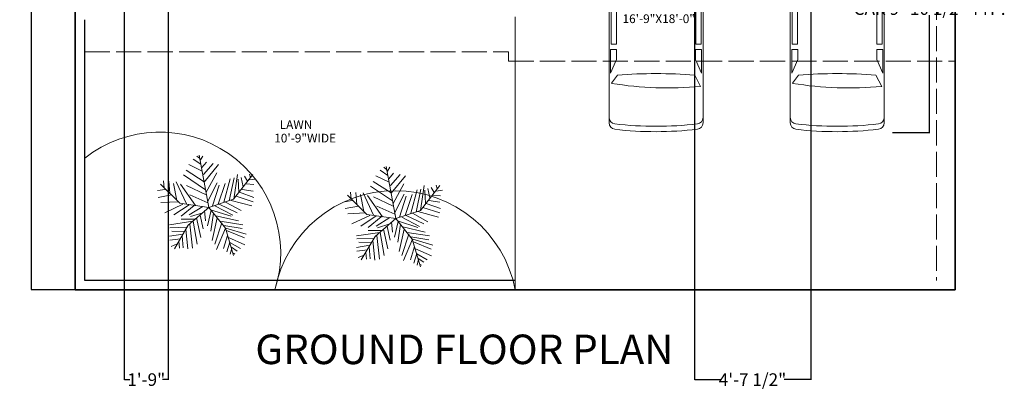
# Model space of a CAD drawing. Units: inches. Extents: x 79 to 8696167, y -3690578 to 147.
# Tile 1 of 10: x 107 to 577, y -732 to -551. Entities that reach past the tile are written whole.
import ezdxf

# ---------------------------------------------------------------- set-up
doc = ezdxf.new("R2010")
doc.units = ezdxf.units.IN
doc.header["$MEASUREMENT"] = 0
doc.linetypes.add('ACAD_ISO02W100', pattern=[15, 12, -3])
doc.layers.get('0').update_dxf_attribs({"color": 253})
for name, color, linetype, lineweight in [('A-ANNO-DIMS', 2, 'Continuous', 18), ('A-AREA-IDEN', 7, 'Continuous', 18), ('A-FLOR-PROJ', 8, 'ACAD_ISO02W100', 13), ('C-PKNG-VEHI', 8, 'Continuous', 13), ('C-PROP', 7, 'Continuous', 35), ('C-SITE-WALL', 8, 'Continuous', 25), ('garden', 114, 'Continuous', 18), ('PLUMBING FIXTURES', 9, 'Continuous', 18), ('text', 7, 'Continuous', 18)]:
    doc.layers.add(name, color=color, linetype=linetype, lineweight=lineweight)
doc.styles.get("Standard").update_dxf_attribs({"font": 'arial.ttf'})
doc.dimstyles.get("Standard").update_dxf_attribs({"dimtxt": 6, "dimasz": 0.18, "dimexe": 0.18, "dimexo": 0.0625, "dimgap": 0.09, "dimtad": 0, "dimtih": 1, "dimtoh": 1, "dimzin": 0, "dimdsep": 46, "dimlunit": 3, "dimtxsty": 'Standard', "dimcen": 0.09, "dimadec": 0, "dimazin": 0, "dimtfac": 1, "dimtofl": 0, "dimtmove": 0, "dimatfit": 3, "dimfxl": 1, "dimtolj": 1, "dimtzin": 0, "dimarcsym": 0})

# ---------------------------------------------------------------- blocks, each defined once
blk = doc.blocks.new('CAR')
at = {"layer": 'PLUMBING FIXTURES', "ltscale": 3}
for p, q in [((220804.47, -93720.06), (220804.47, -93547.3)), ((220876.86, -93720.06), (220876.86, -93547.35)), ((220870.5, -93584.17), (220875, -93575.44)), ((220810.83, -93584.17), (220806.31, -93577.76)), ((220810.23, -93596.08), (220805.58, -93585.68)), ((220805.58, -93585.68), (220805.58, -93603.85)), ((220871.11, -93596.08), (220875.75, -93585.68)), ((220875.75, -93585.68), (220875.75, -93603.85)), ((220810.23, -93603.85), (220810.23, -93596.08)), ((220871.11, -93603.85), (220871.11, -93596.08)), ((220805.58, -93603.85), (220810.23, -93603.85)), ((220875.75, -93603.85), (220871.11, -93603.85)), ((220805.99, -93608.09), (220810.13, -93608.09)), ((220805.99, -93653.29), (220805.99, -93608.09)), ((220810.13, -93608.09), (220810.13, -93642.08)), ((220875.35, -93608.09), (220871.21, -93608.09)), ((220871.21, -93608.09), (220871.21, -93642.08)), ((220875.35, -93653.29), (220875.35, -93608.09)), ((220810.13, -93642.08), (220805.99, -93653.29)), ((220871.21, -93642.08), (220875.35, -93653.29)), ((220806.3, -93664.61), (220809.78, -93651.39)), ((220814.66, -93647.63), (220866.67, -93647.63)), ((220875.03, -93664.61), (220871.56, -93651.39)), ((220798.82, -93653.49), (220798.11, -93655.1)), ((220882.52, -93653.49), (220883.22, -93655.1))]:
    blk.add_line(p, q, dxfattribs=at)
for centre, radius, start, end in [((220809.52, -93547.3), 5.05, 97.35661, 179.99999), ((220809.52, -93551.44), 5.05, 97.35661, 179.99999), ((220840.49, -93811.75), 271.3, 83.23106, 96.6925), ((220840.49, -93815.88), 271.3, 83.23106, 96.6925), ((220871.81, -93547.35), 5.05, 359.99999, 82.55935), ((220871.81, -93551.49), 5.05, 359.99999, 82.55935), ((220849.45, -93836.99), 262.8, 84.42019, 99.44802), ((220840.67, -93184.08), 401.19, 265.73533, 274.26465), ((220814.66, -93652.68), 5.05, 89.99999, 165.25643), ((220866.67, -93652.68), 5.05, 14.74356, 89.99999), ((220809.44, -93651.03), 12.03, 199.79435, 245.64582), ((220804.88, -93649.65), 7.17, 212.34744, 266.77131), ((220876.46, -93649.65), 7.17, 273.22867, 327.65255), ((220871.9, -93651.03), 12.03, 294.35417, 340.20564), ((220811.18, -93665.89), 5.05, 165.25643, 260.06484), ((220870.15, -93665.89), 5.05, 279.93514, 14.74356), ((220840.67, -93484.81), 188.52, 260.73418, 279.2658), ((220809.52, -93714.44), 5.05, 179.99999, 251.46365), ((220809.52, -93720.06), 5.05, 179.99999, 252.55068), ((220840.67, -93611.64), 112.45, 253.06746, 286.93252), ((220871.81, -93720.06), 5.05, 287.4493, 359.99999), ((220871.81, -93714.44), 5.05, 288.53634, 359.99999), ((220840.67, -93610.47), 118.98, 254.06731, 285.93267)]:
    blk.add_arc(centre, radius, start, end, dxfattribs=at)
blk = doc.blocks.new('*U21')
for p, q in [((-10.186, 53.64), (-13.084, 55.962)), ((0, 0), (-10.5, 57)), ((-9.099, 51.782), (-6.563, 55.962)), ((-7.288, 39.707), (-21.778, 46.673)), ((-8.737, 47.138), (-17.069, 52.711)), ((-7.65, 43.423), (-2.578, 49.46)), ((-5.839, 35.992), (4.667, 48.067)), ((-5.114, 27.632), (10.463, 46.673)), ((-3.665, 19.273), (-27.574, 35.527)), ((-5.114, 28.097), (-24.676, 40.636)), ((-2.941, 16.486), (8.652, 37.85)), ((22.055, 7.198), (27.489, 32.277)), ((27, 9), (48, 36)), ((27.127, 9.056), (31.112, 35.992)), ((35.096, 32.741), (37.27, 22.524)), ((38.719, 34.134), (41.979, 28.561)), ((44.153, 36.456), (45.239, 32.741)), ((-31.5, 4.5), (-52.5, 25.5)), ((-48.585, 21.131), (-49.309, 29.026)), ((-43.513, 28.561), (-42.427, 15.558)), ((-38.442, 26.239), (-34.819, 7.663)), ((-35.544, 28.097), (-24.314, 3.947)), ((-14.533, 2.09), (-30.834, 25.31)), ((-24.314, 23.917), (-2.941, 13.7)), ((-1.129, 6.734), (9.014, 26.704)), ((3.942, 1.625), (11.187, 24.381)), ((10.101, 3.483), (17.708, 26.239)), ((16.259, 5.805), (23.142, 31.348)), ((31.836, 30.883), (32.561, 16.486)), ((40.53, 25.775), (48.862, 24.846)), ((43.791, 29.954), (51.036, 30.883)), ((-47.498, 19.737), (-55.83, 18.344)), ((-40.615, 13.7), (-55.105, 10.913)), ((-20.691, 13.7), (-1.129, 4.876)), ((29.662, 12.307), (48.137, 6.269)), ((33.285, 16.486), (48.862, 10.913)), ((36.183, 19.737), (48.137, 17.88)), ((-33.37, 6.269), (-52.207, 5.34)), ((-28.299, 3.483), (-47.86, -5.805)), ((-21.416, 3.018), (-38.079, -8.128)), ((0, 0), (-31.5, 4.5)), ((-15.982, 2.09), (-30.11, -9.521)), ((0, 0), (-22.5, -19.5)), ((-6.563, 1.161), (-21.416, -8.128)), ((0, 0), (27, 9)), ((0, 0), (18, -22.5)), ((6.478, 1.625), (26.04, -8.592)), ((11.187, 3.483), (30.749, -5.805)), ((18.07, 5.805), (35.096, -3.483)), ((24.229, 7.663), (46.688, 1.625)), ((-6.563, -5.805), (-19.967, -9.985)), ((-9.461, -8.592), (-6.201, -23.453)), ((-4.752, -3.483), (-3.665, -14.629)), ((2.493, -3.019), (-1.491, -20.202)), ((1.769, -2.555), (24.229, -9.521)), ((5.029, -6.27), (2.131, -25.775)), ((7.565, -9.056), (32.198, -14.629)), ((-17.431, -15.094), (-42.789, -18.809)), ((-22.5, -19.5), (-37.5, -45)), ((-15.257, -12.772), (-30.11, -12.772)), ((-20.691, -18.345), (-17.793, -44.352)), ((-17.069, -15.094), (-12.721, -40.172)), ((-13.446, -11.378), (-8.737, -32.741)), ((9.014, -11.378), (3.58, -35.992)), ((14.085, -16.951), (6.478, -40.172)), ((12.274, -15.094), (36.907, -18.809)), ((16.259, -19.738), (36.183, -22.989)), ((-28.299, -29.026), (-42.789, -31.348)), ((-24.314, -21.596), (-42.427, -22.06)), ((-26.849, -26.24), (-40.253, -25.775)), ((-29.023, -30.884), (-27.936, -43.887)), ((-25.038, -23.918), (-22.865, -45.281)), ((18.07, -22.524), (8.289, -45.745)), ((20.244, -30.419), (15.897, -44.816)), ((18, -22.5), (27, -52.5)), ((18.433, -22.524), (40.53, -29.026)), ((19.157, -25.311), (38.719, -33.206)), ((-30.834, -34.135), (-42.427, -35.528)), ((-34.457, -39.708), (-40.978, -42.494)), ((-32.646, -36.921), (-31.921, -44.352)), ((22.78, -37.85), (19.519, -48.532)), ((21.331, -32.741), (39.081, -40.636)), ((22.78, -38.314), (34.372, -44.816)), ((24.591, -45.745), (23.142, -50.854)), ((24.591, -43.423), (30.749, -47.603)), ((26.764, -49.925), (28.213, -50.854))]:
    blk.add_line(p, q)
blk = doc.blocks.new('*D23')
at = {"layer": 'A-ANNO-DIMS', "color": 0, "lineweight": -2, "transparency": 16777216}
for p, q in [((133.38, 99.88), (112.4, 99.88)), ((112.58, 99.7), (112.58, -286.97)), ((112.58, -679.94), (112.58, -293.28)), ((133.38, -680.12), (112.4, -680.12))]:
    blk.add_line(p, q, dxfattribs=at)
at = {"layer": 'A-ANNO-DIMS', "color": 0, "lineweight": 100, "transparency": 16777216}
for points in [[(112.55, 99.7), (112.61, 99.7), (112.58, 99.88)], [(112.55, -679.94), (112.61, -679.94), (112.58, -680.12)]]:
    blk.add_solid(points, dxfattribs=at)
at = {"layer": 'Defpoints', "color": 0, "lineweight": 100, "transparency": 16777216}
for p in [(112.58, 99.88), (133.44, 99.88), (133.44, -680.12)]:
    blk.add_point(p, dxfattribs=at)
at = {"layer": 'A-ANNO-DIMS', "color": 0, "transparency": 16777216, "insert": (112.58, -290.12), "char_height": 6, "attachment_point": 5}
blk.add_mtext("\\A1;65'", dxfattribs=at)
blk = doc.blocks.new('*D53')
at = {"layer": 'A-ANNO-DIMS', "color": 0, "lineweight": -2, "transparency": 16777216}
for p, q in [((523.51, -486.61), (541.38, -486.61)), ((541.2, -486.79), (541.2, -542.6)), ((541.2, -604.78), (541.2, -548.98)), ((523.51, -604.96), (541.38, -604.96))]:
    blk.add_line(p, q, dxfattribs=at)
at = {"layer": 'A-ANNO-DIMS', "color": 0, "lineweight": 100, "transparency": 16777216}
for points in [[(541.17, -486.79), (541.23, -486.79), (541.2, -486.61)], [(541.17, -604.78), (541.23, -604.78), (541.2, -604.96)]]:
    blk.add_solid(points, dxfattribs=at)
at = {"layer": 'Defpoints', "color": 0, "lineweight": 100, "transparency": 16777216}
for p in [(523.45, -486.61), (523.45, -604.96), (541.2, -604.96)]:
    blk.add_point(p, dxfattribs=at)
at = {"layer": 'A-ANNO-DIMS', "color": 0, "transparency": 16777216, "insert": (541.2, -545.79), "char_height": 6, "attachment_point": 5}
blk.add_mtext('\\A1;CAR 9\'-10 1/2" TYP.', dxfattribs=at)
blk = doc.blocks.new('*D57')
at = {"layer": 'A-ANNO-DIMS', "color": 0, "lineweight": -2, "transparency": 16777216}
for p, q in [((428.94, -155.06), (428.94, -723.2)), ((484.44, -155.06), (484.44, -723.2)), ((429.12, -723.02), (441.51, -723.02)), ((484.26, -723.02), (471.87, -723.02))]:
    blk.add_line(p, q, dxfattribs=at)
at = {"layer": 'A-ANNO-DIMS', "color": 0, "lineweight": 100, "transparency": 16777216}
for points in [[(429.12, -722.99), (429.12, -723.05), (428.94, -723.02)], [(484.26, -722.99), (484.26, -723.05), (484.44, -723.02)]]:
    blk.add_solid(points, dxfattribs=at)
at = {"layer": 'Defpoints', "color": 0, "lineweight": 100, "transparency": 16777216}
for p in [(428.94, -155), (484.44, -155), (484.44, -723.02)]:
    blk.add_point(p, dxfattribs=at)
at = {"layer": 'A-ANNO-DIMS', "color": 0, "transparency": 16777216, "insert": (456.69, -723.02), "char_height": 6, "attachment_point": 5}
blk.add_mtext('\\A1;4\'-7 1/2"', dxfattribs=at)
blk = doc.blocks.new('*D59')
at = {"layer": 'A-ANNO-DIMS', "color": 0, "lineweight": -2, "transparency": 16777216}
for p, q in [((156.82, 2.31), (156.82, -723.2)), ((177.82, 2.31), (177.82, -723.2)), ((157, -723.02), (159.53, -723.02)), ((177.64, -723.02), (175.1, -723.02))]:
    blk.add_line(p, q, dxfattribs=at)
at = {"layer": 'A-ANNO-DIMS', "color": 0, "lineweight": 100, "transparency": 16777216}
for points in [[(157, -722.99), (157, -723.05), (156.82, -723.02)], [(177.64, -722.99), (177.64, -723.05), (177.82, -723.02)]]:
    blk.add_solid(points, dxfattribs=at)
at = {"layer": 'Defpoints', "color": 0, "lineweight": 100, "transparency": 16777216}
for p in [(156.82, 2.38), (177.82, 2.38), (177.82, -723.02)]:
    blk.add_point(p, dxfattribs=at)
at = {"layer": 'A-ANNO-DIMS', "color": 0, "transparency": 16777216, "insert": (167.32, -723.02), "char_height": 6, "attachment_point": 5}
blk.add_mtext('\\A1;1\'-9"', dxfattribs=at)

msp = doc.modelspace()

# ---------------------------------------------------------------- linework, layer by layer
at = {"layer": 'A-FLOR-PROJ'}
for p, q in [((544.441, -464.125), (544.441, -675.625)), ((137.941, -566.494), (340.24, -566.494)), ((340.24, -566.494), (340.24, -570.943)), ((340.24, -570.943), (553.441, -570.943))]:
    msp.add_line(p, q, dxfattribs=at)
at = {"layer": 'C-PROP'}
for p, q in [((133.441, -680.125), (133.441, 99.875)), ((553.441, 99.875), (553.441, -680.125)), ((553.441, -680.125), (133.441, -680.125))]:
    msp.add_line(p, q, dxfattribs=at)
at = {"layer": 'C-SITE-WALL'}
for p, q in [((133.441, -680.125), (133.441, -551.125)), ((137.941, -675.625), (137.941, -551.125)), ((343.441, -675.625), (137.941, -675.625))]:
    msp.add_line(p, q, dxfattribs=at)
at = {"layer": 'garden'}
msp.add_line((343.441, -549.625), (343.441, -680.125), dxfattribs=at)
for centre, radius, start, end in [((173.696, -662.561), 57.788, 342.30556, 128.22422), ((286.095, -691.206), 58.406, 10.93674, 169.06326)]:
    msp.add_arc(centre, radius, start, end, dxfattribs=at)

# ---------------------------------------------------------------- block references
at = {"layer": 'C-PKNG-VEHI', "xscale": -0.6191396643141144, "yscale": 0.6191396643141144, "zscale": 0.6191396643141144, "rotation": 180}
for p in [(-136320.559, -58519.176), (-136234.115, -58519.176)]:
    msp.add_blockref('CAR', p, dxfattribs=at)
at = {"layer": 'garden', "xscale": 0.4381751191577558, "yscale": 0.4381751191577558, "zscale": 0.4381751191577558}
for p in [(197.187, -640.772), (286.398, -646.124)]:
    msp.add_blockref('*U21', p, dxfattribs=at)

# ---------------------------------------------------------------- texts
at = {"layer": 'A-AREA-IDEN'}
for s, height, p in [('16\'-9"X18\'-0"', 4.15558, (394.627, -552.679)), ('LAWN', 4.1556, (230.979, -603.268)), ('10\'-9"WIDE', 4.1556, (228.379, -609.726))]:
    msp.add_text(s, height=height, dxfattribs=at).set_placement(p)
at = {"layer": 'text'}
msp.add_text('GROUND FLOOR PLAN', height=14.10754, dxfattribs=at).set_placement((219.38, -715.624))

# ---------------------------------------------------------------- dimensions: what is measured, and where the dimension line sits
at = {"layer": 'A-ANNO-DIMS'}
dim = msp.add_linear_dim(base=(112.58, 99.875), p1=(133.441, -680.125), p2=(133.441, 99.875), angle=90, dimstyle='Standard', override={"dimclrd": 0, "dimclre": 0, "dimclrt": 0}, dxfattribs=at)
dim.commit()
dim.dimension.update_dxf_attribs({"geometry": '*D23', "text_midpoint": (112.58, -290.125)})
for base, p1, p2, picture, middle in [((177.817, -723.025), (156.817, 2.375), (177.817, 2.375), '*D59', (167.317, -723.025)), ((484.441, -723.025), (428.941, -154.996), (484.441, -154.996), '*D57', (456.691, -723.025))]:
    dim = msp.add_linear_dim(base=base, p1=p1, p2=p2, dimstyle='Standard', override={"dimdec": 1, "dimlfac": 1, "dimrnd": 0, "dimzin": 1, "dimdsep": 46, "dimlunit": 4, "dimfrac": 2}, dxfattribs=at)
    dim.commit()
    dim.dimension.update_dxf_attribs({"geometry": picture, "text_midpoint": middle})
dim = msp.add_linear_dim(base=(541.202, -604.964), p1=(523.449, -486.613), p2=(523.449, -604.964), angle=270, text='CAR <> TYP.', dimstyle='Standard', override={"dimdec": 1, "dimlfac": 1, "dimrnd": 0, "dimzin": 1, "dimdsep": 46, "dimlunit": 4, "dimfrac": 2}, dxfattribs=at)
dim.commit()
dim.dimension.update_dxf_attribs({"geometry": '*D53', "text_midpoint": (541.202, -545.788)})

doc.saveas('drawing.dxf')
